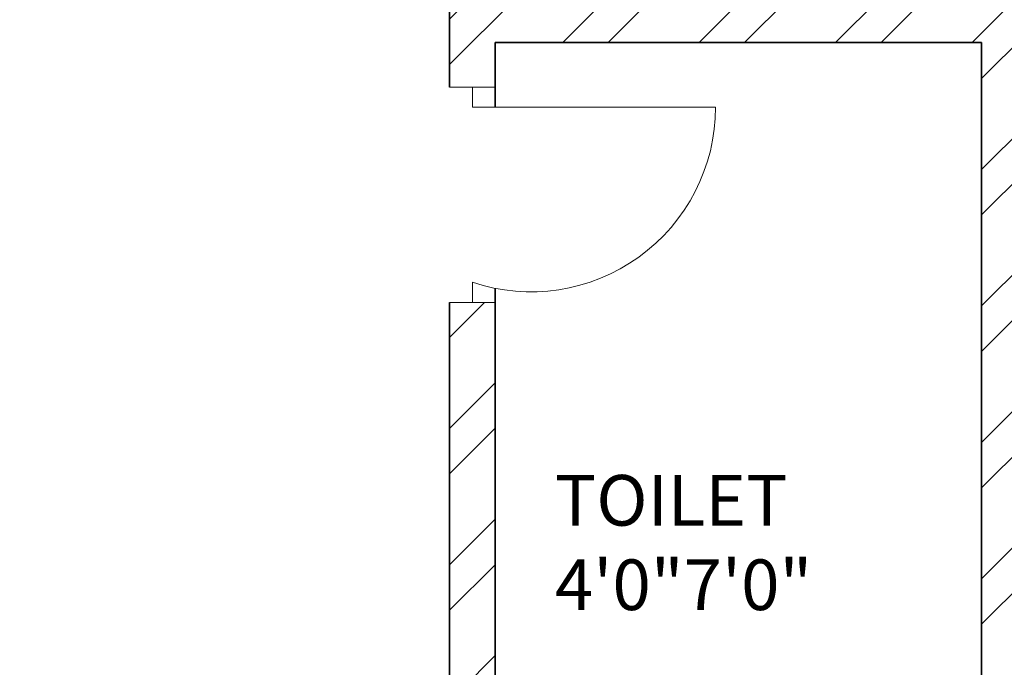
# Model space of a CAD drawing. Units: inches. Extents: x 1885 to 2748, y 783 to 2421.
# Tile 19 of 117: x 2065 to 2163, y 1114 to 1178. Entities that reach past the tile are written whole.
import ezdxf

# ---------------------------------------------------------------- set-up
doc = ezdxf.new("R2010")
doc.units = ezdxf.units.IN
for name, color, linetype, lineweight in [('A-AREA-IDEN', 7, 'Continuous', 18), ('A-DOOR', 31, 'Continuous', 18), ('A-WALL', 7, 'Continuous', 35)]:
    doc.layers.add(name, color=color, linetype=linetype, lineweight=lineweight)
doc.layers.add('A-WALL-PATT', color=85, linetype='Continuous', lineweight=13, true_color=0x58ba48)
doc.styles.get("Standard").update_dxf_attribs({"font": 'arial.ttf'})

msp = doc.modelspace()

# ---------------------------------------------------------------- hatches: boundary and pattern name
at = {"layer": 'A-WALL-PATT'}
h = msp.add_hatch(dxfattribs=at)
h.set_pattern_fill('ANSI32', color=256)
h.paths.add_polyline_path([(2007.772, 2318.006), (1980.774, 2318.006), (1980.774, 2281.215), (1985.274, 2281.215), (1985.274, 2313.506), (2007.772, 2313.506), (2007.772, 2315.756)])
h.paths.add_polyline_path([(2094.324, 2318.006), (2067.772, 2318.006), (2067.772, 2313.506), (2094.324, 2313.506), (2094.324, 2315.756)])
h.paths.add_polyline_path([(2131.367, 2315.756), (2131.367, 2318.006), (2131.189, 2318.006), (2112.609, 2318.006), (2112.609, 2313.506), (2117.274, 2313.506), (2117.274, 2255.201), (2121.774, 2255.201), (2121.774, 2313.506), (2131.367, 2313.506)])
h.paths.add_polyline_path([(2190.512, 2318.006), (2155.367, 2318.006), (2155.367, 2313.506), (2169.774, 2313.506), (2169.774, 2229.506), (2121.774, 2229.506), (2121.774, 2233.451), (2119.524, 2233.451), (2117.274, 2233.451), (2117.274, 2201.101), (2121.774, 2201.101), (2121.774, 2225.006), (2169.774, 2225.006), (2169.774, 2165.006), (2306.274, 2165.006), (2306.274, 2066.006), (2310.774, 2066.006), (2344.274, 2066.006), (2486.274, 2066.006), (2486.274, 1886.006), (2483.02, 1886.006), (2483.02, 1881.506), (2486.274, 1881.506), (2486.274, 1880.678), (2490.774, 1880.678), (2490.774, 2070.506), (2344.274, 2070.506), (2310.774, 2070.506), (2310.774, 2165.006), (2310.774, 2173.636), (2308.524, 2173.636), (2306.274, 2173.636), (2306.274, 2169.506), (2174.274, 2169.506), (2174.274, 2313.506), (2190.512, 2313.506), (2190.512, 2315.756)])
h.paths.add_polyline_path([(1985.274, 2221.215), (1980.774, 2221.215), (1980.774, 2165.006), (1992.774, 2165.006), (1992.774, 2141.927), (1997.274, 2141.927), (1997.274, 2165.006), (2117.274, 2165.006), (2117.274, 2163.126), (2121.774, 2163.126), (2121.774, 2172.734), (2119.524, 2172.734), (2117.274, 2172.734), (2117.274, 2169.506), (1985.274, 2169.506)])
h.paths.add_polyline_path([(1997.274, 2105.927), (1992.774, 2105.927), (1992.774, 2070.506), (2016.774, 2070.506), (2016.774, 2059.123), (2019.024, 2059.123), (2021.274, 2059.123), (2021.274, 2070.506), (2117.274, 2070.506), (2117.274, 2022.506), (2114.423, 2022.506), (2114.423, 2018.006), (2123.627, 2018.006), (2123.627, 2020.256), (2123.627, 2022.506), (2121.774, 2022.506), (2121.774, 2142.587), (2119.524, 2142.587), (2117.274, 2142.587), (2117.274, 2075.006), (1997.274, 2075.006)])
h.paths.add_polyline_path([(2092.029, 2020.256), (2092.029, 2022.506), (2021.274, 2022.506), (2021.274, 2035.123), (2016.774, 2035.123), (2016.774, 2018.006), (2016.774, 1978.784), (2021.274, 1978.784), (2021.274, 2018.006), (2092.029, 2018.006)])
h.paths.add_polyline_path([(2260.938, 2022.506), (2153.105, 2022.506), (2153.105, 2020.256), (2153.105, 2018.006), (2155.274, 2018.006), (2155.274, 1886.006), (2107.629, 1886.006), (2107.629, 1881.506), (2182.911, 1881.506), (2182.911, 1883.756), (2182.911, 1886.006), (2159.774, 1886.006), (2159.774, 2018.006), (2260.938, 2018.006), (2260.938, 2020.256)])
h.paths.add_polyline_path([(2047.629, 1883.756), (2047.629, 1886.006), (2021.274, 1886.006), (2021.274, 1918.784), (2019.024, 1918.784), (2016.774, 1918.784), (2016.774, 1881.506), (2047.629, 1881.506)])
h.paths.add_polyline_path([(2306.361, 1883.756), (2306.361, 1886.006), (2296.274, 1886.006), (2296.274, 1982.006), (2316.535, 1982.006), (2316.535, 1984.256), (2316.535, 1986.506), (2296.274, 1986.506), (2296.274, 2022.506), (2289.276, 2022.506), (2289.276, 2018.006), (2291.774, 2018.006), (2291.774, 1886.006), (2242.911, 1886.006), (2242.911, 1881.506), (2306.361, 1881.506)], flags=17)
h.paths.add_polyline_path([(1985.274, 1843.006), (2021.6, 1843.006), (2021.534, 1845.441), (2021.477, 1847.506), (1980.774, 1847.506), (1980.774, 1809.446), (1985.274, 1809.446)])
h.paths.add_polyline_path([(2131.482, 1845.256), (2131.482, 1847.506), (2081.534, 1847.506), (2081.534, 1843.006), (2117.274, 1843.006), (2117.274, 1784.147), (2119.524, 1784.147), (2121.774, 1784.147), (2121.774, 1843.006), (2131.482, 1843.006)])
h.paths.add_polyline_path([(2203.886, 1847.506), (2155.482, 1847.506), (2155.482, 1843.006), (2169.774, 1843.006), (2169.774, 1759.006), (2121.774, 1759.006), (2121.774, 1761.457), (2117.274, 1761.457), (2117.274, 1730.429), (2121.774, 1730.429), (2121.774, 1754.506), (2177.421, 1754.506), (2177.421, 1756.756), (2177.421, 1759.006), (2174.274, 1759.006), (2174.274, 1843.006), (2203.886, 1843.006)])
h.paths.add_polyline_path([(2335.554, 1845.256), (2335.554, 1847.506), (2239.886, 1847.506), (2239.886, 1843.006), (2306.274, 1843.006), (2306.274, 1759.006), (2199.486, 1759.006), (2199.486, 1754.506), (2310.774, 1754.506), (2310.774, 1843.006), (2335.554, 1843.006)])
h.paths.add_polyline_path([(2348.774, 2022.506), (2344.274, 2022.506), (2344.274, 1986.506), (2341.681, 1986.506), (2341.681, 1982.006), (2344.274, 1982.006), (2344.274, 1886.006), (2330.361, 1886.006), (2330.361, 1881.506), (2361.627, 1881.506), (2361.627, 1883.756), (2361.627, 1886.006), (2348.774, 1886.006)], flags=17)
h.paths.add_polyline_path([(2283.251, 2315.756), (2283.251, 2318.006), (2238.512, 2318.006), (2238.512, 2313.506), (2283.251, 2313.506)], flags=17)
h.paths.add_polyline_path([(2363.274, 2348.006), (2388.677, 2348.006), (2388.677, 2350.256), (2388.677, 2352.506), (2358.774, 2352.506), (2358.774, 2348.006), (2358.774, 2318.006), (2344.481, 2318.006), (2344.481, 2313.506), (2358.774, 2313.506), (2358.774, 2229.506), (2310.774, 2229.506), (2310.774, 2231.952), (2306.274, 2231.952), (2306.274, 2205.611), (2310.774, 2205.611), (2310.774, 2225.006), (2358.774, 2225.006), (2358.774, 2211.506), (2452.329, 2211.506), (2452.329, 2213.756), (2452.329, 2216.006), (2363.274, 2216.006), (2363.274, 2318.006)])
h.paths.add_polyline_path([(2310.774, 2313.506), (2320.481, 2313.506), (2320.481, 2315.756), (2320.481, 2318.006), (2302.728, 2318.006), (2302.728, 2313.506), (2306.274, 2313.506), (2306.274, 2251.076), (2310.774, 2251.076)], flags=17)
h.paths.add_polyline_path([(2490.774, 2352.506), (2486.274, 2352.506), (2448.677, 2352.506), (2448.677, 2348.006), (2486.274, 2348.006), (2486.274, 2318.006), (2486.274, 2216.006), (2481.78, 2216.006), (2481.78, 2211.506), (2486.274, 2211.506), (2486.274, 2165.006), (2493.289, 2165.006), (2493.289, 2167.256), (2493.289, 2169.506), (2490.774, 2169.506), (2490.774, 2313.506), (2494.429, 2313.506), (2494.429, 2318.006), (2490.774, 2318.006)])
h.paths.add_polyline_path([(2534.653, 2318.006), (2515.691, 2318.006), (2515.691, 2313.506), (2534.653, 2313.506), (2534.653, 2315.756)])
h.paths.add_polyline_path([(2618.274, 2318.006), (2594.653, 2318.006), (2594.653, 2313.506), (2613.774, 2313.506), (2613.774, 2281.706), (2618.274, 2281.706)])
h.paths.add_polyline_path([(2618.274, 2221.706), (2613.774, 2221.706), (2613.774, 2169.506), (2554.019, 2169.506), (2554.019, 2165.006), (2613.774, 2165.006), (2613.774, 2152.878), (2618.274, 2152.878)])
h.paths.add_polyline_path([(2618.274, 2128.878), (2616.024, 2128.878), (2613.774, 2128.878), (2613.774, 2117.006), (2529.774, 2117.006), (2529.774, 2165.006), (2532.848, 2165.006), (2532.848, 2169.506), (2522.867, 2169.506), (2522.867, 2165.006), (2525.274, 2165.006), (2525.274, 2117.006), (2525.274, 2112.506), (2525.274, 2108.576), (2529.774, 2108.576), (2529.774, 2112.506), (2613.774, 2112.506), (2613.774, 2080.19), (2618.274, 2080.19)])
h.paths.add_polyline_path([(2618.274, 2044.19), (2616.024, 2044.19), (2613.774, 2044.19), (2613.774, 2015.506), (2529.774, 2015.506), (2529.774, 2088.582), (2527.524, 2088.582), (2525.274, 2088.582), (2525.274, 2011.006), (2613.774, 2011.006), (2613.774, 1956.755), (2618.274, 1956.755)])
h.paths.add_polyline_path([(2618.274, 1881.506), (2618.274, 1896.755), (2613.774, 1896.755), (2613.774, 1881.506), (2613.774, 1847.506), (2592.715, 1847.506), (2592.715, 1843.006), (2613.774, 1843.006), (2613.774, 1765.006), (2613.774, 1760.506), (2609.621, 1760.506), (2609.621, 1756.006), (2613.774, 1756.006), (2613.774, 1660.006), (2608.544, 1660.006), (2608.544, 1655.506), (2613.774, 1655.506), (2613.774, 1508.158), (2618.274, 1508.158)])
h.paths.add_polyline_path([(2565.774, 1843.006), (2568.997, 1843.006), (2568.997, 1847.506), (2490.774, 1847.506), (2490.774, 1849.7), (2488.524, 1849.7), (2486.274, 1849.7), (2486.274, 1847.506), (2477.274, 1847.506), (2477.274, 1838.506), (2477.274, 1821.493), (2486.274, 1821.493), (2486.274, 1838.506), (2561.274, 1838.506), (2561.274, 1765.006), (2486.274, 1765.006), (2486.274, 1786.157), (2477.274, 1786.157), (2477.274, 1765.006), (2477.274, 1756.006), (2486.274, 1756.006), (2565.774, 1756.006), (2585.621, 1756.006), (2585.621, 1758.256), (2585.621, 1760.506), (2565.774, 1760.506), (2565.774, 1765.006)])
h.paths.add_polyline_path([(2486.274, 1651.006), (2561.274, 1651.006), (2561.274, 1567.006), (2486.274, 1567.006), (2486.274, 1591.321), (2477.274, 1591.321), (2477.274, 1567.006), (2477.274, 1558.006), (2477.274, 1555.439), (2481.774, 1555.439), (2481.774, 1558.006), (2568.653, 1558.006), (2568.653, 1560.256), (2568.653, 1562.506), (2565.774, 1562.506), (2565.774, 1655.506), (2584.544, 1655.506), (2584.544, 1657.756), (2584.544, 1660.006), (2565.774, 1660.006), (2486.274, 1660.006), (2477.274, 1660.006), (2477.274, 1651.006), (2477.274, 1632.989), (2486.274, 1632.989)])
h.paths.add_polyline_path([(2449.967, 1883.756), (2449.967, 1886.006), (2421.627, 1886.006), (2421.627, 1881.506), (2449.967, 1881.506)], flags=17)
h.paths.add_polyline_path([(2447.274, 1847.506), (2395.554, 1847.506), (2395.554, 1843.006), (2442.774, 1843.006), (2442.774, 1809.27), (2447.274, 1809.27)])
h.paths.add_polyline_path([(1985.274, 1749.446), (1980.774, 1749.446), (1980.774, 1694.504), (1985.274, 1694.504), (1985.274, 1694.506), (1986.897, 1694.506), (1986.897, 1697.78), (1986.897, 1699.006), (1985.274, 1699.006)])
h.paths.add_polyline_path([(2152.774, 1699.006), (2121.774, 1699.006), (2121.774, 1703.668), (2119.524, 1703.668), (2117.274, 1703.668), (2117.274, 1699.006), (2009.219, 1699.006), (2009.219, 1694.506), (2148.274, 1694.506), (2148.274, 1692.631), (2152.774, 1692.631)])
h.paths.add_polyline_path([(2016.274, 1694.506), (2011.774, 1694.506), (2011.774, 1558.006), (2040.806, 1558.006), (2040.806, 1560.256), (2040.806, 1562.506), (2016.274, 1562.506)])
h.paths.add_polyline_path([(2152.774, 1663.017), (2150.524, 1663.017), (2148.274, 1663.017), (2148.274, 1562.506), (2100.806, 1562.506), (2100.806, 1558.006), (2165.119, 1558.006), (2165.119, 1560.256), (2165.119, 1562.506), (2152.774, 1562.506), (2152.774, 1610.506), (2224.774, 1610.506), (2224.774, 1607.99), (2229.274, 1607.99), (2229.274, 1615.006), (2152.774, 1615.006)])
h.paths.add_polyline_path([(2238.613, 1560.256), (2238.613, 1562.506), (2229.274, 1562.506), (2229.274, 1588.756), (2227.024, 1588.763), (2224.774, 1588.771), (2224.774, 1562.506), (2189.119, 1562.506), (2189.119, 1558.006), (2238.613, 1558.006)])
h.paths.add_polyline_path([(2336.024, 1560.256), (2336.024, 1562.506), (2310.774, 1562.506), (2310.774, 1656.347), (2308.524, 1656.347), (2306.274, 1656.347), (2306.274, 1562.506), (2286.613, 1562.506), (2286.613, 1558.006), (2336.024, 1558.006)])
h.paths.add_polyline_path([(2447.274, 1690.968), (2445.024, 1690.968), (2442.774, 1690.968), (2442.774, 1687.006), (2306.274, 1687.006), (2306.274, 1680.75), (2310.774, 1680.75), (2310.774, 1682.506), (2442.774, 1682.506), (2442.774, 1562.506), (2396.024, 1562.506), (2396.024, 1558.006), (2447.274, 1558.006)])
h.paths.add_polyline_path([(2447.274, 1749.27), (2445.024, 1749.27), (2442.774, 1749.27), (2442.774, 1717.232), (2447.274, 1717.232)])
h.paths.add_polyline_path([(2044.674, 1521.756), (2044.674, 1524.006), (2007.274, 1524.006), (2007.274, 1503.49), (2009.524, 1503.49), (2011.774, 1503.49), (2011.774, 1519.506), (2044.674, 1519.506)])
h.paths.add_polyline_path([(2177.969, 1521.756), (2177.969, 1524.006), (2104.674, 1524.006), (2104.674, 1519.506), (2145.774, 1519.506), (2145.774, 1387.506), (2143.37, 1387.506), (2143.37, 1383.006), (2251.585, 1383.006), (2251.585, 1385.256), (2251.585, 1387.506), (2150.274, 1387.506), (2150.274, 1519.506), (2177.969, 1519.506)])
h.paths.add_polyline_path([(2298.704, 1524.006), (2237.969, 1524.006), (2237.969, 1519.506), (2282.274, 1519.506), (2282.274, 1387.506), (2279.683, 1387.506), (2279.683, 1383.006), (2286.774, 1383.006), (2286.774, 1419.006), (2312.451, 1419.006), (2312.451, 1421.256), (2312.451, 1423.506), (2286.774, 1423.506), (2286.774, 1519.506), (2298.704, 1519.506), (2298.704, 1521.722)], flags=17)
h.paths.add_polyline_path([(2361.897, 1521.756), (2361.897, 1524.006), (2322.704, 1524.006), (2322.704, 1519.506), (2334.774, 1519.506), (2334.774, 1423.506), (2331.93, 1423.506), (2331.93, 1419.006), (2334.774, 1419.006), (2334.774, 1387.506), (2334.774, 1383.228), (2339.274, 1383.228), (2339.274, 1387.506), (2339.274, 1519.506), (2361.897, 1519.506)], flags=17)
h.paths.add_polyline_path([(2447.274, 1521.756), (2447.274, 1524.006), (2421.897, 1524.006), (2421.897, 1519.506), (2447.274, 1519.506)], flags=17)
h.paths.add_polyline_path([(2481.774, 1529.6), (2479.524, 1529.6), (2477.274, 1529.6), (2477.274, 1524.006), (2474.489, 1524.006), (2474.489, 1519.506), (2477.274, 1519.506), (2477.274, 1334.506), (2296.774, 1334.506), (2296.774, 1240.506), (2160.274, 1240.506), (2160.274, 1180.506), (2112.274, 1180.506), (2112.274, 1207.692), (2110.024, 1207.692), (2107.774, 1207.692), (2107.774, 1171.609), (2112.274, 1171.609), (2112.274, 1176.006), (2160.274, 1176.006), (2160.274, 1092.006), (2144.221, 1092.006), (2144.221, 1087.506), (2189.497, 1087.506), (2189.497, 1089.756), (2189.497, 1092.006), (2164.774, 1092.006), (2164.774, 1236.006), (2296.774, 1236.006), (2296.774, 1231.912), (2301.274, 1231.912), (2301.274, 1330.006), (2481.774, 1330.006), (2481.774, 1387.506)])
h.paths.add_polyline_path([(2618.274, 1448.158), (2613.774, 1448.158), (2613.774, 1382.506), (2529.774, 1382.506), (2525.274, 1382.506), (2525.274, 1307.062), (2529.774, 1307.062), (2529.774, 1378.006), (2613.774, 1378.006), (2613.774, 1354.988), (2618.274, 1354.988)])
h.paths.add_polyline_path([(2618.274, 1318.988), (2613.774, 1318.988), (2613.774, 1281.006), (2529.774, 1281.006), (2529.774, 1283.786), (2527.524, 1283.786), (2525.274, 1283.786), (2525.274, 1228.506), (2516.794, 1228.506), (2516.794, 1224.006), (2533.484, 1224.006), (2533.484, 1226.256), (2533.484, 1228.506), (2529.774, 1228.506), (2529.774, 1276.506), (2613.774, 1276.506), (2613.774, 1266.02), (2618.274, 1266.02)])
h.paths.add_polyline_path([(2618.274, 1134.964), (2613.774, 1134.964), (2613.774, 1092.006), (2594.545, 1092.006), (2594.545, 1087.506), (2618.274, 1087.506)])
h.paths.add_polyline_path([(2534.545, 1092.006), (2509.765, 1092.006), (2509.765, 1087.506), (2534.545, 1087.506), (2534.545, 1089.756)])
h.paths.add_polyline_path([(2481.274, 1224.006), (2484.117, 1224.006), (2484.117, 1226.256), (2484.117, 1228.506), (2476.774, 1228.506), (2476.774, 1198.506), (2471.61, 1198.506), (2471.61, 1194.006), (2476.774, 1194.006), (2476.774, 1062.006), (2436.894, 1062.006), (2436.894, 1057.506), (2476.774, 1057.506), (2481.274, 1057.506), (2481.274, 1062.006), (2481.274, 1087.506), (2485.354, 1087.506), (2485.354, 1089.756), (2485.354, 1092.006), (2481.274, 1092.006), (2481.274, 1117.506)])
h.paths.add_polyline_path([(2439.898, 1198.506), (2349.274, 1198.506), (2349.274, 1194.006), (2349.274, 1180.506), (2301.274, 1180.506), (2301.274, 1201.896), (2299.024, 1201.896), (2296.774, 1201.896), (2296.774, 1172.335), (2299.024, 1172.335), (2301.274, 1172.335), (2301.274, 1176.006), (2349.274, 1176.006), (2349.274, 1092.006), (2334.452, 1092.006), (2334.452, 1087.506), (2349.274, 1087.506), (2349.274, 1057.506), (2353.774, 1057.506), (2376.894, 1057.506), (2376.894, 1059.756), (2376.894, 1062.006), (2353.774, 1062.006), (2353.774, 1087.506), (2353.774, 1180.506), (2353.774, 1194.006), (2439.898, 1194.006), (2439.898, 1196.256)])
h.paths.add_polyline_path([(2270.596, 1089.756), (2270.596, 1092.006), (2249.497, 1092.006), (2249.497, 1087.506), (2270.596, 1087.506)], flags=17)
h.paths.add_polyline_path([(2310.452, 1092.006), (2301.274, 1092.006), (2301.274, 1153.292), (2296.774, 1153.292), (2296.774, 1092.006), (2293.786, 1092.006), (2293.786, 1087.506), (2310.452, 1087.506), (2310.452, 1089.756)], flags=17)
h.paths.add_polyline_path([(2112.274, 1150.328), (2110.024, 1150.328), (2107.774, 1150.328), (2107.774, 1092.006), (2104.465, 1092.006), (2104.465, 1087.506), (2120.221, 1087.506), (2120.221, 1089.756), (2120.221, 1092.006), (2112.274, 1092.006)])
h.paths.add_polyline_path([(2082.172, 1092.006), (2058.144, 1092.006), (2058.144, 1087.506), (2082.172, 1087.506), (2082.172, 1089.756)])
h.paths.add_polyline_path([(1975.774, 1145.638), (1971.274, 1145.638), (1971.274, 1087.506), (1980.774, 1087.506), (1998.144, 1087.506), (1998.144, 1089.756), (1998.144, 1092.006), (1985.274, 1092.006), (1975.774, 1092.006)])
h.paths.add_polyline_path([(2112.274, 1244.385), (2110.024, 1244.385), (2107.774, 1244.385), (2107.774, 1240.506), (1992.274, 1240.506), (1992.274, 1271.008), (1987.774, 1271.008), (1987.774, 1240.506), (1980.774, 1240.506), (1975.774, 1240.506), (1971.274, 1240.506), (1971.274, 1205.638), (1975.774, 1205.638), (1975.774, 1236.006), (2107.774, 1236.006), (2107.774, 1233.444), (2112.274, 1233.444), (2112.274, 1236.006)])
h.paths.add_polyline_path([(2112.274, 1383.006), (2114.783, 1383.006), (2114.783, 1385.256), (2114.783, 1387.506), (2102.476, 1387.506), (2102.476, 1383.006), (2107.774, 1383.006), (2107.774, 1335.006), (2011.774, 1335.006), (2011.774, 1349.939), (2007.274, 1349.939), (2007.274, 1335.006), (1987.774, 1335.006), (1987.774, 1330.506), (1987.774, 1307.008), (1992.274, 1307.008), (1992.274, 1330.506), (2007.274, 1330.506), (2107.774, 1330.506), (2107.774, 1264.711), (2112.274, 1264.711)])
h.paths.add_polyline_path([(2077.857, 1387.506), (2011.774, 1387.506), (2011.774, 1390.036), (2009.524, 1390.036), (2007.274, 1390.036), (2007.274, 1373.939), (2011.774, 1373.939), (2011.774, 1383.006), (2077.857, 1383.006)])
h.paths.add_polyline_path([(2011.774, 1443.49), (2007.274, 1443.49), (2007.274, 1410.248), (2011.774, 1410.248)])

# ---------------------------------------------------------------- linework, layer by layer
at = {"layer": 'A-DOOR'}
for p, q in [((2107.774, 1171.609), (2112.274, 1171.609)), ((2112.274, 1171.609), (2110.024, 1171.609)), ((2110.024, 1171.609), (2110.024, 1169.609)), ((2110.024, 1169.609), (2134.024, 1169.609)), ((2110.024, 1150.328), (2110.024, 1152.328)), ((2107.774, 1150.328), (2112.274, 1150.328)), ((2112.274, 1150.328), (2110.024, 1150.328))]:
    msp.add_line(p, q, dxfattribs=at)
msp.add_arc((2115.802, 1169.609), 18.221, 251.50984, 360, dxfattribs=at)
at = {"layer": 'A-WALL'}
for p, q in [((2107.774, 1171.609), (2107.774, 1208.651)), ((2160.274, 1176.006), (2112.274, 1176.006)), ((2112.274, 1176.006), (2112.274, 1169.609)), ((2160.274, 1176.006), (2160.274, 1092.006)), ((2112.274, 1151.733), (2112.274, 1092.006)), ((2107.774, 1092.006), (2107.774, 1150.328))]:
    msp.add_line(p, q, dxfattribs=at)

# ---------------------------------------------------------------- texts
at = {"layer": 'A-AREA-IDEN', "insert": (2118.164, 1133.299), "char_height": 5, "attachment_point": 1}
msp.add_mtext_dynamic_manual_height_columns('TOILET\\P4\'0"7\'0"', width=106.5292, gutter_width=12.5, heights=[0], dxfattribs=at)

doc.saveas('drawing.dxf')
